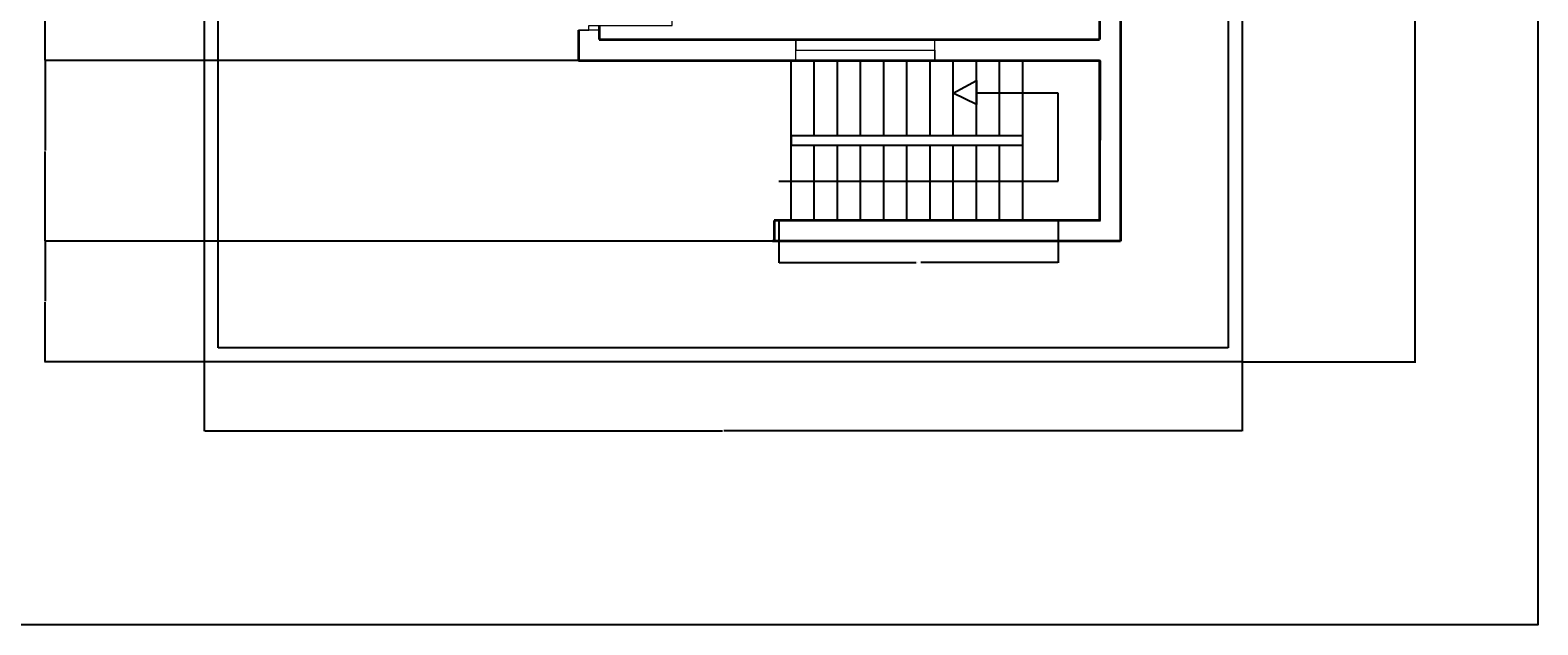
# Model space of a CAD drawing. Units: inches. Extents: x 1587 to 2880, y 1287 to 2423.
# Tile 6 of 8: x 2229 to 2880, y 1287 to 1543. Entities that reach past the tile are written whole.
import ezdxf

# ---------------------------------------------------------------- set-up
doc = ezdxf.new("R2010")
doc.units = ezdxf.units.IN
for name, color, linetype, lineweight in [('A-ANNO-DIMS', 2, 'Continuous', 18), ('A-ANNO-TTLB', 7, 'Continuous', 25), ('A-DOOR', 3, 'Continuous', 18), ('A-FLOR-STRS', 7, 'Continuous', 25), ('A-GLAZ', 4, 'Continuous', 18), ('A-WALL', 7, 'Continuous', 35), ('C-PROP', 8, 'Continuous', 25)]:
    doc.layers.add(name, color=color, linetype=linetype, lineweight=lineweight)
doc.styles.get("Standard").update_dxf_attribs({"font": 'arial.ttf'})
doc.dimstyles.get("Standard").update_dxf_attribs({"dimtxt": 0.18, "dimasz": 0.18, "dimexe": 0.18, "dimexo": 0.0625, "dimgap": 0.09, "dimtad": 0, "dimtih": 1, "dimtoh": 1, "dimdec": 4, "dimzin": 0, "dimdsep": 46, "dimtxsty": 'Standard', "dimcen": 0.09, "dimadec": 0, "dimazin": 0, "dimtfac": 1, "dimtdec": 4, "dimtofl": 0, "dimtmove": 0, "dimatfit": 3, "dimfxl": 1, "dimtolj": 1, "dimtzin": 0, "dimarcsym": 0})

# ---------------------------------------------------------------- blocks, each defined once
blk = doc.blocks.new('WIN-60IN')
for p, q in [((0, 60), (9, 60)), ((9, 60), (4.5, 60)), ((4.5, 60), (4.5, 0)), ((4.5, 0), (0, 0)), ((0, 0), (9, 0))]:
    blk.add_line(p, q)
blk = doc.blocks.new('DOOR-36IN-ENTRY')
for p, q in [((0, 31.08), (9, 31.08)), ((4.5, 31.08), (4.5, 29.08)), ((9, 0), (0, 0)), ((0, 0), (4.5, 0)), ((4.5, 0), (4.5, 2)), ((4.5, 2), (40.5, 2))]:
    blk.add_line(p, q)
blk.add_arc((12.32, 2), 28.18, 0, 106.09946)
blk = doc.blocks.new('STAIR-RETURN-PLAN')
for p, q in [((5.28, 0), (5.28, 69)), ((15.28, 36.5), (15.28, 69)), ((25.28, 36.5), (25.28, 69)), ((35.28, 36.5), (35.28, 69)), ((45.28, 36.5), (45.28, 69)), ((55.28, 36.5), (55.28, 69)), ((65.28, 36.5), (65.28, 69)), ((75.28, 36.5), (75.28, 69)), ((85.28, 36.5), (85.28, 69)), ((95.28, 36.5), (95.28, 69)), ((105.28, 0), (105.28, 69)), ((75.28, 54.89), (85.28, 60.34)), ((85.28, 60.34), (85.28, 50.05)), ((85.28, 50.05), (75.28, 54.89)), ((120.58, 54.89), (85.28, 54.89)), ((120.58, 16.92), (120.58, 54.89)), ((105.28, 36.5), (5.28, 36.5)), ((5.28, 36.5), (5.28, 34.5)), ((5.28, 34.5), (5.28, 32.5)), ((105.28, 34.5), (105.28, 36.5)), ((5.28, 32.5), (105.28, 32.5)), ((15.28, 0), (15.28, 32.5)), ((25.28, 0), (25.28, 32.5)), ((35.28, 0), (35.28, 32.5)), ((45.28, 0), (45.28, 32.5)), ((55.28, 0), (55.28, 32.5)), ((65.28, 0), (65.28, 32.5)), ((75.28, 0), (75.28, 32.5)), ((85.28, 0), (85.28, 32.5)), ((95.28, 0), (95.28, 32.5)), ((0, 16.92), (120.58, 16.92))]:
    blk.add_line(p, q)
blk = doc.blocks.new('*D39')
at = {"layer": 'A-ANNO-DIMS', "color": 0, "lineweight": -2, "transparency": 16777216}
for p, q in [((2552.54, 1461.32), (2552.54, 1443.12)), ((2673.13, 1461.32), (2673.13, 1443.12)), ((2552.72, 1443.3), (2611.83, 1443.3)), ((2672.95, 1443.3), (2613.84, 1443.3))]:
    blk.add_line(p, q, dxfattribs=at)
at = {"layer": 'A-ANNO-DIMS', "color": 0, "transparency": 16777216}
for points in [[(2552.72, 1443.33), (2552.72, 1443.27), (2552.54, 1443.3)], [(2672.95, 1443.33), (2672.95, 1443.27), (2673.13, 1443.3)]]:
    blk.add_solid(points, dxfattribs=at)
at = {"layer": 'Defpoints', "color": 0, "transparency": 16777216}
for p in [(2552.54, 1461.39), (2673.13, 1461.39), (2673.13, 1443.3)]:
    blk.add_point(p, dxfattribs=at)
at = {"layer": 'A-ANNO-DIMS', "color": 0, "transparency": 16777216, "insert": (2612.83, 1443.3), "char_height": 0.18, "attachment_point": 5}
blk.add_mtext('\\A1;STAIR 121 TYP.', dxfattribs=at)
blk = doc.blocks.new('*D40')
at = {"layer": 'A-ANNO-DIMS', "color": 0, "lineweight": -2, "transparency": 16777216}
for p, q in [((2673.19, 1530.39), (2691.39, 1530.39)), ((2691.21, 1530.21), (2691.21, 1496.07)), ((2691.21, 1461.57), (2691.21, 1495.7)), ((2673.19, 1461.39), (2691.39, 1461.39))]:
    blk.add_line(p, q, dxfattribs=at)
at = {"layer": 'A-ANNO-DIMS', "color": 0, "transparency": 16777216}
for points in [[(2691.18, 1530.21), (2691.24, 1530.21), (2691.21, 1530.39)], [(2691.18, 1461.57), (2691.24, 1461.57), (2691.21, 1461.39)]]:
    blk.add_solid(points, dxfattribs=at)
at = {"layer": 'Defpoints', "color": 0, "transparency": 16777216}
for p in [(2673.13, 1530.39), (2691.21, 1530.39), (2673.13, 1461.39)]:
    blk.add_point(p, dxfattribs=at)
at = {"layer": 'A-ANNO-DIMS', "color": 0, "transparency": 16777216, "insert": (2691.21, 1495.89), "char_height": 0.18, "attachment_point": 5}
blk.add_mtext('\\A1;69 TYP.', dxfattribs=at)
blk = doc.blocks.new('*D45')
at = {"layer": 'A-ANNO-DIMS', "color": 0, "lineweight": -2, "transparency": 16777216}
for p, q in [((2304.53, 1400.32), (2304.53, 1370.46)), ((2752.53, 1400.32), (2752.53, 1370.46)), ((2304.71, 1370.64), (2528.24, 1370.64)), ((2752.35, 1370.64), (2528.83, 1370.64))]:
    blk.add_line(p, q, dxfattribs=at)
at = {"layer": 'A-ANNO-DIMS', "color": 0, "transparency": 16777216}
for points in [[(2304.71, 1370.67), (2304.71, 1370.61), (2304.53, 1370.64)], [(2752.35, 1370.67), (2752.35, 1370.61), (2752.53, 1370.64)]]:
    blk.add_solid(points, dxfattribs=at)
at = {"layer": 'Defpoints', "color": 0, "transparency": 16777216}
for p in [(2304.53, 1400.39), (2752.53, 1400.39), (2752.53, 1370.64)]:
    blk.add_point(p, dxfattribs=at)
at = {"layer": 'A-ANNO-DIMS', "color": 0, "transparency": 16777216, "insert": (2528.53, 1370.64), "char_height": 0.18, "attachment_point": 5}
blk.add_mtext('\\A1;448', dxfattribs=at)
blk = doc.blocks.new('*D46')
at = {"layer": 'A-ANNO-DIMS', "color": 0, "lineweight": -2, "transparency": 16777216}
for p, q in [((2752.6, 1988.39), (2827.47, 1988.39)), ((2827.29, 1988.21), (2827.29, 1694.57)), ((2827.29, 1400.57), (2827.29, 1694.2)), ((2752.6, 1400.39), (2827.47, 1400.39))]:
    blk.add_line(p, q, dxfattribs=at)
at = {"layer": 'A-ANNO-DIMS', "color": 0, "transparency": 16777216}
for points in [[(2827.26, 1988.21), (2827.32, 1988.21), (2827.29, 1988.39)], [(2827.26, 1400.57), (2827.32, 1400.57), (2827.29, 1400.39)]]:
    blk.add_solid(points, dxfattribs=at)
at = {"layer": 'Defpoints', "color": 0, "transparency": 16777216}
for p in [(2752.53, 1988.39), (2827.29, 1988.39), (2752.53, 1400.39)]:
    blk.add_point(p, dxfattribs=at)
at = {"layer": 'A-ANNO-DIMS', "color": 0, "transparency": 16777216, "insert": (2827.29, 1694.39), "char_height": 0.18, "attachment_point": 5}
blk.add_mtext('\\A1;588', dxfattribs=at)
blk = doc.blocks.new('*D56')
at = {"layer": 'A-ANNO-DIMS', "color": 0, "lineweight": -2, "transparency": 16777216}
for p, q in [((2550.42, 1452.39), (2235.59, 1452.39)), ((2235.77, 1452.21), (2235.77, 1426.57)), ((2235.77, 1400.57), (2235.77, 1426.2)), ((2304.47, 1400.39), (2235.59, 1400.39))]:
    blk.add_line(p, q, dxfattribs=at)
at = {"layer": 'A-ANNO-DIMS', "color": 0, "transparency": 16777216}
for points in [[(2235.74, 1452.21), (2235.8, 1452.21), (2235.77, 1452.39)], [(2235.74, 1400.57), (2235.8, 1400.57), (2235.77, 1400.39)]]:
    blk.add_solid(points, dxfattribs=at)
at = {"layer": 'Defpoints', "color": 0, "transparency": 16777216}
for p in [(2550.49, 1452.39), (2235.77, 1400.39), (2304.53, 1400.39)]:
    blk.add_point(p, dxfattribs=at)
at = {"layer": 'A-ANNO-DIMS', "color": 0, "transparency": 16777216, "insert": (2235.77, 1426.39), "char_height": 0.18, "attachment_point": 5}
blk.add_mtext('\\A1;52', dxfattribs=at)
blk = doc.blocks.new('*D57')
at = {"layer": 'A-ANNO-DIMS', "color": 0, "lineweight": -2, "transparency": 16777216}
for p, q in [((2465.97, 1530.39), (2235.59, 1530.39)), ((2235.77, 1530.21), (2235.77, 1491.57)), ((2235.77, 1452.57), (2235.77, 1491.2)), ((2550.42, 1452.39), (2235.59, 1452.39))]:
    blk.add_line(p, q, dxfattribs=at)
at = {"layer": 'A-ANNO-DIMS', "color": 0, "transparency": 16777216}
for points in [[(2235.74, 1530.21), (2235.8, 1530.21), (2235.77, 1530.39)], [(2235.74, 1452.57), (2235.8, 1452.57), (2235.77, 1452.39)]]:
    blk.add_solid(points, dxfattribs=at)
at = {"layer": 'Defpoints', "color": 0, "transparency": 16777216}
for p in [(2466.03, 1530.39), (2235.77, 1452.39), (2550.49, 1452.39)]:
    blk.add_point(p, dxfattribs=at)
at = {"layer": 'A-ANNO-DIMS', "color": 0, "transparency": 16777216, "insert": (2235.77, 1491.39), "char_height": 0.18, "attachment_point": 5}
blk.add_mtext('\\A1;78', dxfattribs=at)
blk = doc.blocks.new('*D58')
at = {"layer": 'A-ANNO-DIMS', "color": 0, "lineweight": -2, "transparency": 16777216}
for p, q in [((2341.47, 1578.89), (2235.59, 1578.89)), ((2235.77, 1578.71), (2235.77, 1554.82)), ((2235.77, 1530.57), (2235.77, 1554.45)), ((2465.97, 1530.39), (2235.59, 1530.39))]:
    blk.add_line(p, q, dxfattribs=at)
at = {"layer": 'A-ANNO-DIMS', "color": 0, "transparency": 16777216}
for points in [[(2235.74, 1578.71), (2235.8, 1578.71), (2235.77, 1578.89)], [(2235.74, 1530.57), (2235.8, 1530.57), (2235.77, 1530.39)]]:
    blk.add_solid(points, dxfattribs=at)
at = {"layer": 'Defpoints', "color": 0, "transparency": 16777216}
for p in [(2235.77, 1578.89), (2341.53, 1578.89), (2466.03, 1530.39)]:
    blk.add_point(p, dxfattribs=at)
at = {"layer": 'A-ANNO-DIMS', "color": 0, "transparency": 16777216, "insert": (2235.77, 1554.64), "char_height": 0.18, "attachment_point": 5}
blk.add_mtext('\\A1;48.5', dxfattribs=at)

msp = doc.modelspace()

# ---------------------------------------------------------------- linework, layer by layer
at = {"layer": 'A-ANNO-TTLB'}
msp.add_lwpolyline([(1586.5185, 2423.1539), (2880.2062, 2423.1539), (2880.2062, 1286.9347), (1586.5185, 1286.9347)], close=True, dxfattribs=at)
at = {"layer": 'A-WALL'}
for p, q in [((2700.034, 1788.9874), (2700.034, 1530.3868)), ((2691.034, 1695.3868), (2691.034, 1539.3868)), ((2466.034, 1543.4794), (2466.034, 1530.3868)), ((2475.034, 1545.4794), (2475.034, 1539.3868)), ((2475.034, 1539.3868), (2691.034, 1539.3868)), ((2466.034, 1530.3868), (2691.034, 1530.3868)), ((2691.034, 1530.3868), (2691.034, 1461.3868)), ((2700.034, 1530.3868), (2700.034, 1452.3868)), ((2691.034, 1461.3868), (2550.4857, 1461.3868)), ((2550.4857, 1461.3868), (2550.4857, 1452.3868)), ((2700.034, 1452.3868), (2549.8543, 1452.3868))]:
    msp.add_line(p, q, dxfattribs=at)
at = {"layer": 'C-PROP'}
for p, q in [((2304.534, 1988.3868), (2304.534, 1400.3868)), ((2310.534, 1406.3868), (2310.534, 1988.3868)), ((2746.534, 1886.3868), (2746.534, 1406.3868)), ((2752.534, 1886.3868), (2752.534, 1400.3868)), ((2746.534, 1406.3868), (2310.534, 1406.3868)), ((2752.534, 1400.3868), (2304.534, 1400.3868))]:
    msp.add_line(p, q, dxfattribs=at)

# ---------------------------------------------------------------- block references
at = {"layer": 'A-DOOR'}
msp.add_blockref('DOOR-36IN-ENTRY', (2466.034, 1543.4794), dxfattribs=at)
at = {"layer": 'A-FLOR-STRS'}
msp.add_blockref('STAIR-RETURN-PLAN', (2552.5418, 1461.3868), dxfattribs=at)
at = {"layer": 'A-GLAZ', "rotation": 89.99999999999969}
msp.add_blockref('WIN-60IN', (2619.8512, 1530.3865), dxfattribs=at)

# ---------------------------------------------------------------- dimensions: what is measured, and where the dimension line sits
at = {"layer": 'A-ANNO-DIMS'}
for base, p1, p2, override, picture, middle in [((2827.2911, 1988.3868), (2752.534, 1400.3868), (2752.534, 1988.3868), {"dimdec": 0, "dimlfac": 1, "dimrnd": 0, "dimzin": 0, "dimdsep": 46, "dimlunit": 2}, '*D46', (2827.2911, 1694.3868)), ((2235.766, 1578.8868), (2466.034, 1530.3868), (2341.534, 1578.8868), {"dimdec": 1, "dimlfac": 1, "dimrnd": 0, "dimzin": 0, "dimdsep": 46, "dimlunit": 2}, '*D58', (2235.766, 1554.6368)), ((2235.766, 1452.3868), (2466.034, 1530.3868), (2550.4857, 1452.3868), {"dimdec": 0, "dimlfac": 1, "dimrnd": 0, "dimzin": 0, "dimdsep": 46, "dimlunit": 2}, '*D57', (2235.766, 1491.3868)), ((2235.766, 1400.3868), (2550.4857, 1452.3868), (2304.534, 1400.3868), {"dimdec": 0, "dimlfac": 1, "dimrnd": 0, "dimzin": 0, "dimdsep": 46, "dimlunit": 2}, '*D56', (2235.766, 1426.3868))]:
    dim = msp.add_linear_dim(base=base, p1=p1, p2=p2, angle=90, dimstyle='Standard', override=override, dxfattribs=at)
    dim.commit()
    dim.dimension.update_dxf_attribs({"geometry": picture, "text_midpoint": middle})
dim = msp.add_linear_dim(base=(2691.2127, 1530.3868), p1=(2673.1252, 1461.3868), p2=(2673.1252, 1530.3868), angle=90, text='<> TYP.', dimstyle='Standard', override={"dimdec": 0, "dimlfac": 1, "dimrnd": 0, "dimzin": 0, "dimdsep": 46, "dimlunit": 2}, dxfattribs=at)
dim.commit()
dim.dimension.update_dxf_attribs({"geometry": '*D40', "text_midpoint": (2691.2127, 1495.8868)})
dim = msp.add_linear_dim(base=(2673.1252, 1443.2993), p1=(2552.5418, 1461.3868), p2=(2673.1252, 1461.3868), text='STAIR <> TYP.', dimstyle='Standard', override={"dimdec": 0, "dimlfac": 1, "dimrnd": 0, "dimzin": 0, "dimdsep": 46, "dimlunit": 2}, dxfattribs=at)
dim.commit()
dim.dimension.update_dxf_attribs({"geometry": '*D39', "text_midpoint": (2612.8335, 1443.2993)})
dim = msp.add_linear_dim(base=(2752.534, 1370.6368), p1=(2304.534, 1400.3868), p2=(2752.534, 1400.3868), dimstyle='Standard', override={"dimdec": 0, "dimlfac": 1, "dimrnd": 0, "dimzin": 0, "dimdsep": 46, "dimlunit": 2}, dxfattribs=at)
dim.commit()
dim.dimension.update_dxf_attribs({"geometry": '*D45', "text_midpoint": (2528.534, 1370.6368)})

doc.saveas('drawing.dxf')
